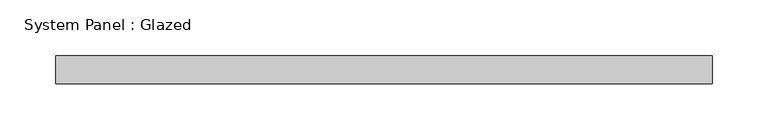
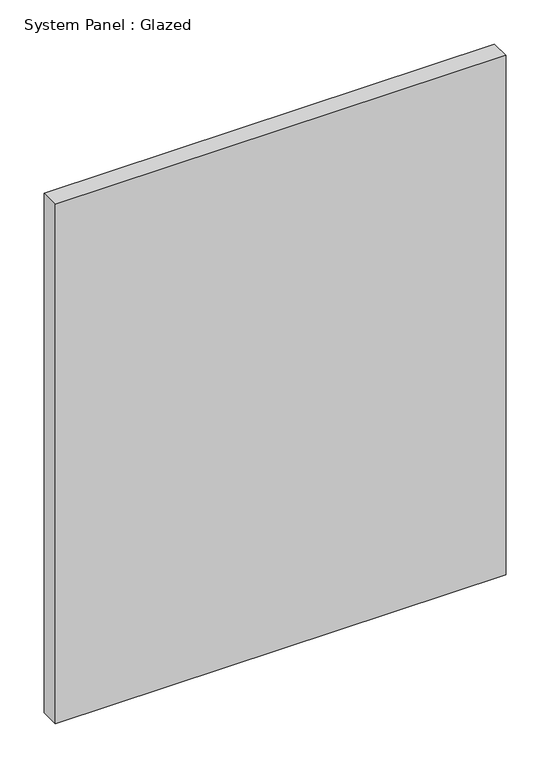
"""IFC4 building model written with IfcOpenShell, lengths in millimetres: plate geometry, System Panel : Glazed."""

from ifc_helpers import new_model, si_unit, origin, origin_with_axes, place, context, project, spatial, polyline, outline, extrude, source, transform, mapped, element, save


def system_panel_glazed_e4ad360d(model_context):
    return source(origin(), model_context, "Body", "SweptSolid", [
        extrude(outline(polyline([(295.275, 19.05), (-295.275, 19.05), (-295.275, 44.45), (295.275, 44.45), (295.275, 19.05)])), origin_with_axes(), (0.0, 0.0, 1.0), 719.3261324),
    ])


if __name__ == "__main__":
    model = new_model("IFC4")
    model_context = context("Model", 3, world=origin())
    ifc_project = project(units=[si_unit("LENGTHUNIT", "METRE", prefix="MILLI")], contexts=[model_context])
    site = spatial("IfcSite", under=ifc_project)
    building = spatial("IfcBuilding", under=site)
    placement = place(None, origin())
    system_panel_glazed_shape = system_panel_glazed_e4ad360d(model_context)
    element("IfcPlate", 1, ObjectType="System Panel : Glazed", at=placement, inside=building, context=model_context, shape_type="MappedRepresentation", body=[
        mapped(system_panel_glazed_shape, transform((0.0, 0.0, 0.0), x_axis=(1.0, 0.0, 0.0), y_axis=(0.0, 1.0, 0.0), z_axis=(0.0, 0.0, 1.0))),
    ])
    save(model, "model.ifc")

# Revit data of these elements
# Type "System Panel : Glazed"
#   Construction Type Id = "GSP4R"
#   Analytic Construction = "1/8 in Pilkington single glazing"
#   Visual Light Transmittance = 0.9
#   Solar Heat Gain Coefficient = 0.86
#   Heat Transfer Coefficient (U) = 1.18115 BTU/(h·ft²·°F)
#   Define Thermal Properties by = 1
# Element 1 (IfcPlate, "System Panel : Glazed")
#   Materials on its faces: "Glass"
# Materials
#   "Glass": class "Glass", colour RGB 0 128 192, transparency 0.75, Description = "Soda Lime Glass", Cost = 0
